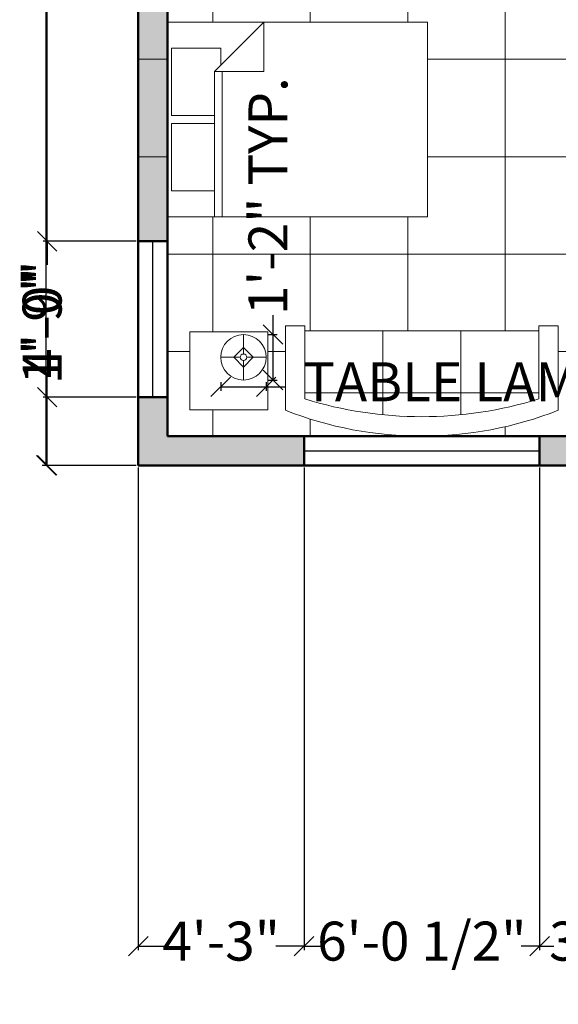
# Model space of a CAD drawing. Units: inches. Extents: x 2371 to 3019, y 129 to 700.
# Tile 1 of 14: x 2371 to 2536, y 129 to 432. Entities that reach past the tile are written whole.
import ezdxf

# ---------------------------------------------------------------- set-up
doc = ezdxf.new("R2010")
doc.units = ezdxf.units.IN
for name, color, linetype, lineweight in [('A-ANNO-DIMS', 2, 'Continuous', 18), ('A-FLOR-PATT', 252, 'Continuous', 13), ('A-FURN', 8, 'Continuous', 18), ('A-GLAZ', 4, 'Continuous', 25), ('A-WALL', 7, 'Continuous', 50), ('A-WALL-PATT', 8, 'Continuous', 13)]:
    doc.layers.add(name, color=color, linetype=linetype, lineweight=lineweight)
doc.styles.get("Standard").update_dxf_attribs({"font": 'arial.ttf'})
doc.dimstyles.new('ISO-25', dxfattribs={"dimtxt": 12, "dimasz": 6, "dimexe": 1.25, "dimexo": 0.625, "dimtad": 0, "dimdec": 1, "dimlunit": 3, "dimtxsty": 'Standard', "dimblk": 'OBLIQUE', "dimblk1": 'ORIGIN2', "dimblk2": 'OBLIQUE', "dimcen": 2.5, "dimadec": 0, "dimazin": 0, "dimtfac": 1, "dimtdec": 1, "dimtmove": 0, "dimatfit": 3, "dimldrblk": 'OBLIQUE', "dimfxl": 1, "dimarcsym": 0})

# ---------------------------------------------------------------- blocks, each defined once
blk = doc.blocks.new('Sofa - Roundback 7 ft.')
for p, q in [((-12.00002, -32.4421), (-12.00003, -6.5971)), ((11.99997, -32.4421), (11.99998, -6.5971)), ((-36.000027, -34), (-36.000027, -11.4696)), ((35.99998, -34), (35.99998, -11.4696)), ((-35.999844, -13.3819), (35.9998, -13.3819)), ((-36.000027, -32.4421), (35.99998, -32.4421))]:
    blk.add_line(p, q)
for points in [[(-36.000027, -34), (-42.000027, -34), (-42.000027, -8)], [(41.99998, -8), (41.99998, -34), (35.99998, -34)]]:
    blk.add_lwpolyline(points)
for centre, radius, start, end in [((0, -114.25), 114.25, 68.43141, 111.5686), ((-0.00001, -127.1968), 121.1968, 72.72033, 107.2797)]:
    blk.add_arc(centre, radius, start, end)
blk = doc.blocks.new('Lamp - Table')
for p, q in [((0, 7), (0, 1)), ((-1, 0), (-7, 0)), ((0, 3), (-3, 0)), ((-3, 0), (0, -3)), ((3, 0), (0, 3)), ((0, -3), (3, 0)), ((1, 0), (7, 0)), ((0, -1), (0, -7))]:
    blk.add_line(p, q)
for radius in [7, 1]:
    blk.add_circle((0, 0), radius)
blk = doc.blocks.new('Bed - Queen')
for p, q in [((0, -80.00003), (0, 0)), ((0, 0), (59.99999, 0)), ((59.99999, 0), (59.99999, -80.00003)), ((7.99999, -1.2), (28.79998, -1.2)), ((7.99999, -14.4), (7.99999, -1.2)), ((28.79998, -1.2), (28.79998, -14.4)), ((31.19999, -1.2), (51.99999, -1.2)), ((31.19999, -14.4), (31.19999, -1.2)), ((51.99999, -1.2), (51.99999, -16.4)), ((0, -14.4), (44.8, -14.4)), ((59.99999, -29.6), (44.8, -14.4)), ((44.8, -14.4), (44.8, -29.6)), ((44.8, -16.8), (0, -16.8)), ((51.99999, -16.4), (46.79936, -16.4)), ((44.8, -29.6), (59.99999, -29.6)), ((59.99999, -80.00003), (0, -80.00003))]:
    blk.add_line(p, q)
blk = doc.blocks.new('_Oblique')
at = {"color": 0, "linetype": 'ByBlock', "lineweight": -2}
blk.add_line((-0.5, -0.5), (0.5, 0.5), dxfattribs=at)
blk = doc.blocks.new('*D18')
at = {"layer": 'A-ANNO-DIMS', "color": 0, "lineweight": -2, "transparency": 16777216}
for p, q in [((2406.48, 630.98), (2377.53, 630.98)), ((2378.78, 630.98), (2378.78, 484.31)), ((2378.78, 294.98), (2378.78, 441.64)), ((2406.48, 294.98), (2377.53, 294.98))]:
    blk.add_line(p, q, dxfattribs=at)
at = {"layer": 'Defpoints', "color": 0, "lineweight": 25, "transparency": 16777216}
for p in [(2407.11, 630.98), (2378.78, 294.98), (2407.11, 294.98)]:
    blk.add_point(p, dxfattribs=at)
at = {"layer": 'A-ANNO-DIMS', "color": 0, "lineweight": -2, "transparency": 16777216, "xscale": 6, "yscale": 6, "zscale": 6}
for p, rotation in [((2378.78, 630.98), 90), ((2378.78, 294.98), 270)]:
    blk.add_blockref('_Oblique', p, dxfattribs=dict(at, rotation=rotation))
at = {"layer": 'A-ANNO-DIMS', "color": 0, "transparency": 16777216, "insert": (2378.78, 462.98), "char_height": 12, "attachment_point": 5, "rotation": 90}
blk.add_mtext('28\'-0"', dxfattribs=at)
blk = doc.blocks.new('_Origin2')
at = {"color": 0, "linetype": 'ByBlock', "lineweight": -2}
blk.add_line((-0.5, 0), (-1, 0), dxfattribs=at)
for radius in [0.5, 0.25]:
    blk.add_circle((0, 0), radius, dxfattribs=at)
blk = doc.blocks.new('*D22')
at = {"layer": 'A-ANNO-DIMS', "color": 0, "lineweight": -2, "transparency": 16777216}
for p, q in [((2432.46, 320.64), (2432.46, 317.92)), ((2432.46, 319.17), (2446.46, 319.17)), ((2446.46, 320.64), (2446.46, 317.92)), ((2446.46, 319.17), (2452.46, 319.17))]:
    blk.add_line(p, q, dxfattribs=at)
at = {"layer": 'Defpoints', "color": 0, "lineweight": 25, "transparency": 16777216}
for p in [(2432.46, 321.27), (2446.46, 321.27), (2446.46, 319.17)]:
    blk.add_point(p, dxfattribs=at)
at = {"layer": 'A-ANNO-DIMS', "color": 0, "lineweight": -2, "transparency": 16777216, "xscale": 6, "yscale": 6, "zscale": 6, "rotation": 180}
blk.add_blockref('_Oblique', (2432.46, 319.17), dxfattribs=at)
at = {"layer": 'A-ANNO-DIMS', "color": 0, "lineweight": -2, "transparency": 16777216, "xscale": 6, "yscale": 6, "zscale": 6}
blk.add_blockref('_Oblique', (2446.46, 319.17), dxfattribs=at)
at = {"layer": 'A-ANNO-DIMS', "color": 0, "transparency": 16777216, "insert": (2543.85, 319.17), "char_height": 12, "attachment_point": 5}
blk.add_mtext('TABLE LAMP 1\'-2" TYP.', dxfattribs=at)
blk = doc.blocks.new('*D23')
at = {"layer": 'A-ANNO-DIMS', "color": 0, "lineweight": -2, "transparency": 16777216}
for p, q in [((2448.56, 335.27), (2448.56, 341.27)), ((2447.08, 335.27), (2449.81, 335.27)), ((2448.56, 321.27), (2448.56, 335.27)), ((2447.08, 321.27), (2449.81, 321.27))]:
    blk.add_line(p, q, dxfattribs=at)
at = {"layer": 'Defpoints', "color": 0, "lineweight": 25, "transparency": 16777216}
for p in [(2446.46, 335.27), (2448.56, 335.27), (2446.46, 321.27)]:
    blk.add_point(p, dxfattribs=at)
at = {"layer": 'A-ANNO-DIMS', "color": 0, "lineweight": -2, "transparency": 16777216, "xscale": 6, "yscale": 6, "zscale": 6}
for p, rotation in [((2448.56, 335.27), 90), ((2448.56, 321.27), 270)]:
    blk.add_blockref('_Oblique', p, dxfattribs=dict(at, rotation=rotation))
at = {"layer": 'A-ANNO-DIMS', "color": 0, "transparency": 16777216, "insert": (2448.56, 377.9), "char_height": 12, "attachment_point": 5, "rotation": 90}
blk.add_mtext('1\'-2" TYP.', dxfattribs=at)
blk = doc.blocks.new('*D50')
at = {"layer": 'A-ANNO-DIMS', "color": 0, "lineweight": -2, "transparency": 16777216}
for p, q in [((2407.11, 294.35), (2407.11, 145.68)), ((2458.11, 294.35), (2458.11, 145.68)), ((2407.11, 146.93), (2415.79, 146.93)), ((2458.11, 146.93), (2449.42, 146.93))]:
    blk.add_line(p, q, dxfattribs=at)
at = {"layer": 'Defpoints', "color": 0, "lineweight": 25, "transparency": 16777216}
for p in [(2407.11, 294.98), (2458.11, 294.98), (2458.11, 146.93)]:
    blk.add_point(p, dxfattribs=at)
at = {"layer": 'A-ANNO-DIMS', "color": 0, "lineweight": -2, "transparency": 16777216, "xscale": 6, "yscale": 6, "zscale": 6, "rotation": 180}
blk.add_blockref('_Oblique', (2407.11, 146.93), dxfattribs=at)
at = {"layer": 'A-ANNO-DIMS', "color": 0, "lineweight": -2, "transparency": 16777216, "xscale": 6, "yscale": 6, "zscale": 6}
blk.add_blockref('_Oblique', (2458.11, 146.93), dxfattribs=at)
at = {"layer": 'A-ANNO-DIMS', "color": 0, "transparency": 16777216, "insert": (2432.61, 146.93), "char_height": 12, "attachment_point": 5}
blk.add_mtext('4\'-3"', dxfattribs=at)
blk = doc.blocks.new('*D51')
at = {"layer": 'A-ANNO-DIMS', "color": 0, "lineweight": -2, "transparency": 16777216}
for p, q in [((2458.11, 294.35), (2458.11, 145.68)), ((2530.61, 294.35), (2530.61, 145.68)), ((2458.11, 146.93), (2463.77, 146.93)), ((2530.61, 146.93), (2524.94, 146.93))]:
    blk.add_line(p, q, dxfattribs=at)
at = {"layer": 'Defpoints', "color": 0, "lineweight": 25, "transparency": 16777216}
for p in [(2458.11, 294.98), (2530.61, 294.98), (2530.61, 146.93)]:
    blk.add_point(p, dxfattribs=at)
at = {"layer": 'A-ANNO-DIMS', "color": 0, "lineweight": -2, "transparency": 16777216, "xscale": 6, "yscale": 6, "zscale": 6, "rotation": 180}
blk.add_blockref('_Oblique', (2458.11, 146.93), dxfattribs=at)
at = {"layer": 'A-ANNO-DIMS', "color": 0, "lineweight": -2, "transparency": 16777216, "xscale": 6, "yscale": 6, "zscale": 6}
blk.add_blockref('_Oblique', (2530.61, 146.93), dxfattribs=at)
at = {"layer": 'A-ANNO-DIMS', "color": 0, "transparency": 16777216, "insert": (2494.36, 146.93), "char_height": 12, "attachment_point": 5}
blk.add_mtext('6\'-0 1/2"', dxfattribs=at)
blk = doc.blocks.new('*D52')
at = {"layer": 'A-ANNO-DIMS', "color": 0, "lineweight": -2, "transparency": 16777216}
for p, q in [((2530.61, 294.35), (2530.61, 145.68)), ((2572.61, 294.35), (2572.61, 145.68)), ((2530.61, 146.93), (2535.03, 146.93)), ((2572.61, 146.93), (2568.18, 146.93))]:
    blk.add_line(p, q, dxfattribs=at)
at = {"layer": 'Defpoints', "color": 0, "lineweight": 25, "transparency": 16777216}
for p in [(2530.61, 294.98), (2572.61, 294.98), (2572.61, 146.93)]:
    blk.add_point(p, dxfattribs=at)
at = {"layer": 'A-ANNO-DIMS', "color": 0, "lineweight": -2, "transparency": 16777216, "xscale": 6, "yscale": 6, "zscale": 6, "rotation": 180}
blk.add_blockref('_Oblique', (2530.61, 146.93), dxfattribs=at)
at = {"layer": 'A-ANNO-DIMS', "color": 0, "lineweight": -2, "transparency": 16777216, "xscale": 6, "yscale": 6, "zscale": 6}
blk.add_blockref('_Oblique', (2572.61, 146.93), dxfattribs=at)
at = {"layer": 'A-ANNO-DIMS', "color": 0, "transparency": 16777216, "insert": (2551.61, 146.93), "char_height": 12, "attachment_point": 5}
blk.add_mtext('3\'-6"', dxfattribs=at)
blk = doc.blocks.new('*D58')
at = {"layer": 'A-ANNO-DIMS', "color": 0, "lineweight": -2, "transparency": 16777216}
for p, q in [((2379.06, 315.98), (2379.06, 321.98)), ((2406.48, 315.98), (2377.81, 315.98)), ((2379.06, 294.98), (2379.06, 315.98)), ((2406.48, 294.98), (2377.81, 294.98))]:
    blk.add_line(p, q, dxfattribs=at)
at = {"layer": 'Defpoints', "color": 0, "lineweight": 25, "transparency": 16777216}
for p in [(2379.06, 315.98), (2407.11, 315.98), (2407.11, 294.98)]:
    blk.add_point(p, dxfattribs=at)
at = {"layer": 'A-ANNO-DIMS', "color": 0, "lineweight": -2, "transparency": 16777216, "xscale": 6, "yscale": 6, "zscale": 6}
for p, rotation in [((2379.06, 315.98), 90), ((2379.06, 294.98), 270)]:
    blk.add_blockref('_Oblique', p, dxfattribs=dict(at, rotation=rotation))
at = {"layer": 'A-ANNO-DIMS', "color": 0, "transparency": 16777216, "insert": (2379.06, 337.99), "char_height": 12, "attachment_point": 5, "rotation": 90}
blk.add_mtext('1\'-9"', dxfattribs=at)
blk = doc.blocks.new('*D59')
at = {"layer": 'A-ANNO-DIMS', "color": 0, "lineweight": -2, "transparency": 16777216}
for p, q in [((2406.48, 363.98), (2377.81, 363.98)), ((2379.06, 363.98), (2379.06, 356.79)), ((2379.06, 315.98), (2379.06, 323.16)), ((2406.48, 315.98), (2377.81, 315.98))]:
    blk.add_line(p, q, dxfattribs=at)
at = {"layer": 'Defpoints', "color": 0, "lineweight": 25, "transparency": 16777216}
for p in [(2379.06, 363.98), (2407.11, 363.98), (2407.11, 315.98)]:
    blk.add_point(p, dxfattribs=at)
at = {"layer": 'A-ANNO-DIMS', "color": 0, "lineweight": -2, "transparency": 16777216, "xscale": 6, "yscale": 6, "zscale": 6}
for p, rotation in [((2379.06, 363.98), 90), ((2379.06, 315.98), 270)]:
    blk.add_blockref('_Oblique', p, dxfattribs=dict(at, rotation=rotation))
at = {"layer": 'A-ANNO-DIMS', "color": 0, "transparency": 16777216, "insert": (2379.06, 339.98), "char_height": 12, "attachment_point": 5, "rotation": 90}
blk.add_mtext('4\'-0"', dxfattribs=at)
blk = doc.blocks.new('*D60')
at = {"layer": 'A-ANNO-DIMS', "color": 0, "lineweight": -2, "transparency": 16777216}
for p, q in [((2406.48, 630.98), (2377.81, 630.98)), ((2379.06, 630.98), (2379.06, 518.81)), ((2379.06, 363.98), (2379.06, 476.14)), ((2406.48, 363.98), (2377.81, 363.98))]:
    blk.add_line(p, q, dxfattribs=at)
at = {"layer": 'Defpoints', "color": 0, "lineweight": 25, "transparency": 16777216}
for p in [(2379.06, 630.98), (2407.11, 630.98), (2407.11, 363.98)]:
    blk.add_point(p, dxfattribs=at)
at = {"layer": 'A-ANNO-DIMS', "color": 0, "lineweight": -2, "transparency": 16777216, "xscale": 6, "yscale": 6, "zscale": 6}
for p, rotation in [((2379.06, 630.98), 90), ((2379.06, 363.98), 270)]:
    blk.add_blockref('_Oblique', p, dxfattribs=dict(at, rotation=rotation))
at = {"layer": 'A-ANNO-DIMS', "color": 0, "transparency": 16777216, "insert": (2379.06, 497.48), "char_height": 12, "attachment_point": 5, "rotation": 90}
blk.add_mtext('22\'-3"', dxfattribs=at)

msp = doc.modelspace()

# ---------------------------------------------------------------- hatches: boundary and pattern name
at = {"layer": 'A-FLOR-PATT'}
h = msp.add_hatch(dxfattribs=at)
h.set_pattern_fill('_USER', color=256, scale=30, pattern_type=0)
h.set_pattern_definition([(0, (0, 0), (0, 30), [])])
h.paths.add_polyline_path([(2913.11, 498.98), (2827.61, 498.98), (2827.61, 531.98), (2832.11, 531.98), (2832.11, 537.98), (2833.61, 537.98), (2833.61, 605.98), (2818.35, 605.98, -1), (2796.86, 605.98), (2781.61, 605.98), (2781.61, 603.98), (2781.61, 533.98), (2757.61, 533.98), (2757.61, 531.98), (2797.61, 531.98), (2797.61, 522.98), (2757.61, 522.98), (2757.61, 516.98), (2754.59, 516.98), (2772.52, 485.76), (2771.01, 484.89), (2770.98, 484.93, -0.097552), (2757.61, 481.1), (2757.61, 422.48), (2837.61, 422.48), (2837.61, 362.48), (2757.61, 362.48), (2757.61, 303.98), (2835.86, 303.98, -0.09439), (2793.86, 311.98), (2793.86, 337.98), (2799.86, 337.98), (2799.86, 336.42), (2871.86, 336.42), (2871.86, 337.98), (2877.86, 337.98), (2877.86, 311.98, -0.09439), (2835.86, 303.98), (2913.11, 303.98), (2913.11, 383.18), (2904.11, 383.18), (2904.11, 419.18), (2913.11, 419.18)])
h.paths.add_polyline_path([(2788.88, 332.88), (2788.88, 308.88), (2764.88, 308.88), (2764.88, 332.88)], flags=16)
h.paths.add_polyline_path([(2788.4, 325.04, -1), (2774.4, 325.04, -1)], flags=0)
h.paths.add_polyline_path([(2781.4, 328.04), (2784.4, 325.04), (2781.4, 322.04), (2778.4, 325.04)], flags=0)
h.paths.add_polyline_path([(2782.4, 325.04, -1), (2780.4, 325.04, -1)], flags=0)
h.paths.add_polyline_path([(2748.61, 480.99), (2754.51, 480.98, 0.119303), (2770.98, 484.93), (2753.07, 516.1), (2754.59, 516.98), (2748.61, 516.98), (2748.61, 539.98), (2712.61, 539.98), (2665.11, 539.98, -0.09439), (2707.11, 531.98), (2707.11, 505.98), (2701.11, 505.98), (2701.11, 507.53), (2629.11, 507.53), (2629.11, 505.98), (2623.11, 505.98), (2623.11, 531.98, -0.09439), (2665.11, 539.98), (2581.61, 539.98), (2581.61, 522.98), (2581.61, 477.98, -0.131044), (2589.61, 507.98), (2615.61, 507.98), (2615.61, 501.98), (2614.05, 501.98), (2614.05, 453.98), (2615.61, 453.98), (2615.61, 447.98), (2589.61, 447.98, -0.131044), (2581.61, 477.98), (2581.61, 432.98), (2572.61, 432.98, 0.119303), (2556.14, 428.99), (2574.12, 397.85), (2572.61, 396.98), (2578.61, 396.98), (2581.61, 396.98), (2581.61, 390.98), (2748.61, 390.98)])
h.paths.add_polyline_path([(2683.1, 447.25), (2652.43, 447.25), (2652.43, 492.22), (2683.1, 492.22)], flags=16)
h.paths.add_polyline_path([(2682.1, 448.25), (2653.43, 448.25), (2653.43, 491.22), (2682.1, 491.22)], flags=0)
h.paths.add_polyline_path([(2613.58, 512.06), (2589.58, 512.06), (2589.58, 536.06), (2613.58, 536.06)], flags=16)
h.paths.add_polyline_path([(2599.1, 528.22, -1), (2613.1, 528.22, -1)], flags=0)
h.paths.add_polyline_path([(2609.1, 528.22), (2606.1, 525.22), (2603.1, 528.22), (2606.1, 531.22)], flags=0)
h.paths.add_polyline_path([(2607.1, 528.22, -1), (2605.1, 528.22, -1)], flags=0)
h.paths.add_polyline_path([(2581.61, 522.98), (2581.61, 621.98), (2572.61, 621.98), (2572.61, 522.98), (2572.61, 500.98), (2565.85, 500.98), (2565.85, 500.15), (2564.82, 500.15), (2561.16, 500.19), (2561.16, 500.17), (2560.13, 500.3), (2560.22, 500.98), (2556.38, 500.98), (2556.43, 500.22), (2555.4, 500.14), (2555.34, 500.98), (2551.07, 500.98), (2551.07, 500.15), (2550.04, 500.15), (2547.64, 500.19), (2547.64, 500.15), (2546.61, 500.15), (2541.79, 500.22), (2540.72, 500.13), (2540.65, 500.98), (2533.37, 500.98), (2533.37, 500.15), (2532.34, 500.15), (2529.13, 500.21), (2529.12, 500.13), (2528.09, 500.22), (2528.16, 500.98), (2523.23, 500.98), (2523.23, 500.15), (2522.2, 500.15), (2519.8, 500.21), (2519.8, 500.15), (2518.77, 500.15), (2514.45, 500.26), (2514.44, 500.14), (2513.41, 500.22), (2513.47, 500.98), (2509.62, 500.98), (2509.71, 500.3), (2508.69, 500.17), (2508.58, 500.98), (2505.03, 500.98), (2505.03, 500.15), (2503.99, 500.15), (2501.07, 500.29), (2501.07, 500.15), (2500.04, 500.15), (2496.44, 500.37), (2496.44, 500.15), (2495.4, 500.15), (2492.55, 500.41), (2492.18, 500.35), (2492.09, 500.98), (2486.11, 500.98), (2486.11, 524.98), (2486.11, 531.98), (2490.61, 531.98), (2490.61, 537.98), (2492.11, 537.98), (2492.11, 605.98), (2476.85, 605.98, -1), (2455.36, 605.98), (2440.11, 605.98), (2440.11, 533.98), (2416.11, 533.98), (2416.11, 605.98), (2416.11, 621.98), (2536.61, 621.98), (2536.61, 630.98), (2407.11, 630.98), (2407.11, 363.98), (2416.11, 363.98), (2416.11, 431.48), (2496.11, 431.48), (2496.11, 371.48), (2416.11, 371.48), (2416.11, 303.98), (2494.36, 303.98, -0.09439), (2452.36, 311.98), (2452.36, 337.98), (2458.36, 337.98), (2458.36, 336.42), (2530.36, 336.42), (2530.36, 337.98), (2536.36, 337.98), (2536.36, 311.98, -0.09439), (2494.36, 303.98), (2572.61, 303.98), (2572.61, 381.98), (2572.61, 396.98), (2554.61, 428.15), (2556.12, 429.03), (2556.14, 428.99, -0.119303), (2572.61, 432.98), (2578.61, 432.98), (2581.61, 432.98)])
h.paths.add_polyline_path([(2450.11, 500.98), (2444.5, 500.98), (2444.44, 500.14), (2443.41, 500.22), (2443.47, 500.98), (2439.62, 500.98), (2439.71, 500.3), (2438.69, 500.17), (2438.58, 500.98), (2435.02, 500.98), (2435.02, 500.15), (2433.99, 500.15), (2433.99, 500.98), (2431.07, 500.98), (2431.07, 500.15), (2430.04, 500.15), (2430.04, 500.98), (2426.43, 500.98), (2426.43, 500.15), (2425.4, 500.15), (2425.4, 500.98), (2423.13, 500.98), (2423.2, 500.5), (2422.18, 500.35), (2422.09, 500.98), (2416.11, 500.98), (2416.11, 524.98), (2416.11, 531.98), (2450.11, 531.98), (2450.11, 522.98)], flags=16)
h.paths.add_polyline_path([(2449.11, 501.98), (2417.11, 501.98), (2417.11, 522.98), (2417.11, 523.98), (2449.11, 523.98)], flags=0)
h.paths.add_polyline_path([(2420.7, 510.73), (2419.36, 520.07), (2420.38, 520.22), (2421.74, 510.73), (2425.4, 510.73), (2425.4, 520.07), (2426.43, 520.07), (2426.43, 510.73), (2430.04, 510.73), (2430.04, 520.07), (2431.07, 520.07), (2431.07, 510.73), (2433.99, 510.73), (2433.99, 520.07), (2435.02, 520.07), (2435.02, 510.73), (2437.35, 510.73), (2436.18, 519.93), (2437.2, 520.06), (2438.39, 510.73), (2444.17, 510.73), (2444.85, 520.08), (2445.88, 520.01), (2445.21, 510.73)], flags=0)
h.paths.add_polyline_path([(2446.94, 336.11), (2446.94, 312.11), (2422.94, 312.11), (2422.94, 336.11)], flags=16)
h.paths.add_polyline_path([(2446.46, 328.27, -1), (2432.46, 328.27, -1)], flags=0)
h.paths.add_polyline_path([(2439.46, 331.27), (2442.46, 328.27), (2439.46, 325.27), (2436.46, 328.27)], flags=0)
h.paths.add_polyline_path([(2440.46, 328.27, -1), (2438.46, 328.27, -1)], flags=0)
h.paths.add_polyline_path([(2816, 444.88), (2866.87, 444.88), (2866.87, 463.54), (2816, 463.54)], flags=24)
h.paths.add_polyline_path([(2794.21, 558.3), (2833.34, 558.3), (2833.34, 576.96), (2794.21, 576.96)], flags=24)
h.paths.add_polyline_path([(2651.69, 411.53), (2711.04, 411.53), (2711.04, 430.19), (2651.69, 430.19)], flags=24)
h.paths.add_polyline_path([(2494.09, 444.88), (2544.97, 444.88), (2544.97, 463.54), (2494.09, 463.54)], flags=24)
h.paths.add_polyline_path([(2444.55, 565.02), (2483.69, 565.02), (2483.69, 583.68), (2444.55, 583.68)], flags=24)
h = msp.add_hatch(dxfattribs=at)
h.set_pattern_fill('_USER', color=256, scale=30, angle=90, pattern_type=0)
h.set_pattern_definition([(90, (0, 0), (-30, 2e-15), [])])
h.paths.add_polyline_path([(2913.11, 498.98), (2827.61, 498.98), (2827.61, 531.98), (2832.11, 531.98), (2832.11, 537.98), (2833.61, 537.98), (2833.61, 605.98), (2818.35, 605.98, -1), (2796.86, 605.98), (2781.61, 605.98), (2781.61, 603.98), (2781.61, 533.98), (2757.61, 533.98), (2757.61, 531.98), (2797.61, 531.98), (2797.61, 522.98), (2757.61, 522.98), (2757.61, 516.98), (2754.59, 516.98), (2772.52, 485.76), (2771.01, 484.89), (2770.98, 484.93, -0.097552), (2757.61, 481.1), (2757.61, 422.48), (2837.61, 422.48), (2837.61, 362.48), (2757.61, 362.48), (2757.61, 303.98), (2835.86, 303.98, -0.09439), (2793.86, 311.98), (2793.86, 337.98), (2799.86, 337.98), (2799.86, 336.42), (2871.86, 336.42), (2871.86, 337.98), (2877.86, 337.98), (2877.86, 311.98, -0.09439), (2835.86, 303.98), (2913.11, 303.98), (2913.11, 383.18), (2904.11, 383.18), (2904.11, 419.18), (2913.11, 419.18)])
h.paths.add_polyline_path([(2788.88, 332.88), (2788.88, 308.88), (2764.88, 308.88), (2764.88, 332.88)], flags=16)
h.paths.add_polyline_path([(2788.4, 325.04, -1), (2774.4, 325.04, -1)], flags=0)
h.paths.add_polyline_path([(2781.4, 328.04), (2784.4, 325.04), (2781.4, 322.04), (2778.4, 325.04)], flags=0)
h.paths.add_polyline_path([(2782.4, 325.04, -1), (2780.4, 325.04, -1)], flags=0)
h.paths.add_polyline_path([(2748.61, 480.99), (2754.51, 480.98, 0.119303), (2770.98, 484.93), (2753.07, 516.1), (2754.59, 516.98), (2748.61, 516.98), (2748.61, 539.98), (2712.61, 539.98), (2665.11, 539.98, -0.09439), (2707.11, 531.98), (2707.11, 505.98), (2701.11, 505.98), (2701.11, 507.53), (2629.11, 507.53), (2629.11, 505.98), (2623.11, 505.98), (2623.11, 531.98, -0.09439), (2665.11, 539.98), (2581.61, 539.98), (2581.61, 522.98), (2581.61, 477.98, -0.131044), (2589.61, 507.98), (2615.61, 507.98), (2615.61, 501.98), (2614.05, 501.98), (2614.05, 453.98), (2615.61, 453.98), (2615.61, 447.98), (2589.61, 447.98, -0.131044), (2581.61, 477.98), (2581.61, 432.98), (2572.61, 432.98, 0.119303), (2556.14, 428.99), (2574.12, 397.85), (2572.61, 396.98), (2578.61, 396.98), (2581.61, 396.98), (2581.61, 390.98), (2748.61, 390.98)])
h.paths.add_polyline_path([(2683.1, 447.25), (2652.43, 447.25), (2652.43, 492.22), (2683.1, 492.22)], flags=16)
h.paths.add_polyline_path([(2682.1, 448.25), (2653.43, 448.25), (2653.43, 491.22), (2682.1, 491.22)], flags=0)
h.paths.add_polyline_path([(2613.58, 512.06), (2589.58, 512.06), (2589.58, 536.06), (2613.58, 536.06)], flags=16)
h.paths.add_polyline_path([(2599.1, 528.22, -1), (2613.1, 528.22, -1)], flags=0)
h.paths.add_polyline_path([(2609.1, 528.22), (2606.1, 525.22), (2603.1, 528.22), (2606.1, 531.22)], flags=0)
h.paths.add_polyline_path([(2607.1, 528.22, -1), (2605.1, 528.22, -1)], flags=0)
h.paths.add_polyline_path([(2581.61, 522.98), (2581.61, 621.98), (2572.61, 621.98), (2572.61, 522.98), (2572.61, 500.98), (2565.85, 500.98), (2565.85, 500.15), (2564.82, 500.15), (2561.16, 500.19), (2561.16, 500.17), (2560.13, 500.3), (2560.22, 500.98), (2556.38, 500.98), (2556.43, 500.22), (2555.4, 500.14), (2555.34, 500.98), (2551.07, 500.98), (2551.07, 500.15), (2550.04, 500.15), (2547.64, 500.19), (2547.64, 500.15), (2546.61, 500.15), (2541.79, 500.22), (2540.72, 500.13), (2540.65, 500.98), (2533.37, 500.98), (2533.37, 500.15), (2532.34, 500.15), (2529.13, 500.21), (2529.12, 500.13), (2528.09, 500.22), (2528.16, 500.98), (2523.23, 500.98), (2523.23, 500.15), (2522.2, 500.15), (2519.8, 500.21), (2519.8, 500.15), (2518.77, 500.15), (2514.45, 500.26), (2514.44, 500.14), (2513.41, 500.22), (2513.47, 500.98), (2509.62, 500.98), (2509.71, 500.3), (2508.69, 500.17), (2508.58, 500.98), (2505.03, 500.98), (2505.03, 500.15), (2503.99, 500.15), (2501.07, 500.29), (2501.07, 500.15), (2500.04, 500.15), (2496.44, 500.37), (2496.44, 500.15), (2495.4, 500.15), (2492.55, 500.41), (2492.18, 500.35), (2492.09, 500.98), (2486.11, 500.98), (2486.11, 524.98), (2486.11, 531.98), (2490.61, 531.98), (2490.61, 537.98), (2492.11, 537.98), (2492.11, 605.98), (2476.85, 605.98, -1), (2455.36, 605.98), (2440.11, 605.98), (2440.11, 533.98), (2416.11, 533.98), (2416.11, 605.98), (2416.11, 621.98), (2536.61, 621.98), (2536.61, 630.98), (2407.11, 630.98), (2407.11, 363.98), (2416.11, 363.98), (2416.11, 431.48), (2496.11, 431.48), (2496.11, 371.48), (2416.11, 371.48), (2416.11, 303.98), (2494.36, 303.98, -0.09439), (2452.36, 311.98), (2452.36, 337.98), (2458.36, 337.98), (2458.36, 336.42), (2530.36, 336.42), (2530.36, 337.98), (2536.36, 337.98), (2536.36, 311.98, -0.09439), (2494.36, 303.98), (2572.61, 303.98), (2572.61, 381.98), (2572.61, 396.98), (2554.61, 428.15), (2556.12, 429.03), (2556.14, 428.99, -0.119303), (2572.61, 432.98), (2578.61, 432.98), (2581.61, 432.98)])
h.paths.add_polyline_path([(2450.11, 500.98), (2444.5, 500.98), (2444.44, 500.14), (2443.41, 500.22), (2443.47, 500.98), (2439.62, 500.98), (2439.71, 500.3), (2438.69, 500.17), (2438.58, 500.98), (2435.02, 500.98), (2435.02, 500.15), (2433.99, 500.15), (2433.99, 500.98), (2431.07, 500.98), (2431.07, 500.15), (2430.04, 500.15), (2430.04, 500.98), (2426.43, 500.98), (2426.43, 500.15), (2425.4, 500.15), (2425.4, 500.98), (2423.13, 500.98), (2423.2, 500.5), (2422.18, 500.35), (2422.09, 500.98), (2416.11, 500.98), (2416.11, 524.98), (2416.11, 531.98), (2450.11, 531.98), (2450.11, 522.98)], flags=16)
h.paths.add_polyline_path([(2449.11, 501.98), (2417.11, 501.98), (2417.11, 522.98), (2417.11, 523.98), (2449.11, 523.98)], flags=0)
h.paths.add_polyline_path([(2420.7, 510.73), (2419.36, 520.07), (2420.38, 520.22), (2421.74, 510.73), (2425.4, 510.73), (2425.4, 520.07), (2426.43, 520.07), (2426.43, 510.73), (2430.04, 510.73), (2430.04, 520.07), (2431.07, 520.07), (2431.07, 510.73), (2433.99, 510.73), (2433.99, 520.07), (2435.02, 520.07), (2435.02, 510.73), (2437.35, 510.73), (2436.18, 519.93), (2437.2, 520.06), (2438.39, 510.73), (2444.17, 510.73), (2444.85, 520.08), (2445.88, 520.01), (2445.21, 510.73)], flags=0)
h.paths.add_polyline_path([(2446.94, 336.11), (2446.94, 312.11), (2422.94, 312.11), (2422.94, 336.11)], flags=16)
h.paths.add_polyline_path([(2446.46, 328.27, -1), (2432.46, 328.27, -1)], flags=0)
h.paths.add_polyline_path([(2439.46, 331.27), (2442.46, 328.27), (2439.46, 325.27), (2436.46, 328.27)], flags=0)
h.paths.add_polyline_path([(2440.46, 328.27, -1), (2438.46, 328.27, -1)], flags=0)
h.paths.add_polyline_path([(2816, 444.88), (2866.87, 444.88), (2866.87, 463.54), (2816, 463.54)], flags=24)
h.paths.add_polyline_path([(2794.21, 558.3), (2833.34, 558.3), (2833.34, 576.96), (2794.21, 576.96)], flags=24)
h.paths.add_polyline_path([(2651.69, 411.53), (2711.04, 411.53), (2711.04, 430.19), (2651.69, 430.19)], flags=24)
h.paths.add_polyline_path([(2494.09, 444.88), (2544.97, 444.88), (2544.97, 463.54), (2494.09, 463.54)], flags=24)
h.paths.add_polyline_path([(2444.55, 565.02), (2483.69, 565.02), (2483.69, 583.68), (2444.55, 583.68)], flags=24)
at = {"layer": 'A-WALL-PATT'}
h = msp.add_hatch(color=256, dxfattribs=at)
h.dxf.hatch_style = 1
h.paths.add_polyline_path([(2536.61, 630.98), (2407.11, 630.98), (2407.11, 363.98), (2416.11, 363.98), (2416.11, 498.98), (2416.11, 522.98), (2416.11, 531.98), (2416.11, 603.98), (2416.11, 621.98), (2536.61, 621.98)])
h.paths.add_polyline_path([(2630.98, 630.98), (2560.61, 630.98), (2560.61, 621.98), (2630.98, 621.98)])
h.paths.add_polyline_path([(2878.11, 630.98), (2699.23, 630.98), (2699.23, 621.98), (2878.11, 621.98)])
h.paths.add_polyline_path([(2496.61, 621.98), (2492.11, 621.98), (2492.11, 569.98), (2496.61, 569.98)], flags=17)
h.paths.add_polyline_path([(2581.61, 621.98), (2572.61, 621.98), (2572.61, 522.98), (2572.61, 498.98), (2572.61, 432.98), (2578.61, 432.98), (2581.61, 432.98), (2581.61, 522.98)])
h.paths.add_polyline_path([(2572.61, 531.98), (2486.11, 531.98), (2486.11, 522.98), (2572.61, 522.98)])
h.paths.add_polyline_path([(2450.11, 531.98), (2440.11, 531.98), (2416.11, 531.98), (2416.11, 522.98), (2450.11, 522.98)], flags=17)
h.paths.add_polyline_path([(2416.11, 315.98), (2407.11, 315.98), (2407.11, 294.98), (2458.11, 294.98), (2458.11, 303.98), (2416.11, 303.98)])
h.paths.add_polyline_path([(2757.61, 303.98), (2530.61, 303.98), (2530.61, 294.98), (2757.61, 294.98)])
h.paths.add_polyline_path([(2581.61, 381.98), (2605.61, 381.98), (2617.61, 381.98), (2617.61, 390.98), (2581.61, 390.98), (2581.61, 396.98), (2572.61, 396.98), (2572.61, 381.98), (2572.61, 303.98), (2581.61, 303.98)])
h.paths.add_polyline_path([(2757.61, 480.98), (2748.61, 480.98), (2748.61, 381.98), (2748.61, 303.98), (2757.61, 303.98), (2757.61, 381.98), (2757.61, 422.48)])
h.paths.add_polyline_path([(2797.61, 531.98), (2757.61, 531.98), (2757.61, 603.98), (2757.61, 621.98), (2748.61, 621.98), (2748.61, 516.99), (2754.59, 516.98), (2757.61, 516.98), (2757.61, 522.98), (2797.61, 522.98)])
h.paths.add_polyline_path([(2913.11, 531.98), (2827.61, 531.98), (2827.61, 522.98), (2913.11, 522.98)])
h.paths.add_polyline_path([(2923.11, 630.98), (2902.11, 630.98), (2902.11, 621.98), (2914.11, 621.98), (2914.11, 363.98), (2923.11, 363.98)])
h.paths.add_polyline_path([(2923.11, 315.98), (2914.11, 315.98), (2914.11, 303.98), (2866.11, 303.98), (2866.11, 294.98), (2923.11, 294.98)])
h.paths.add_polyline_path([(2793.61, 303.98), (2757.61, 303.98), (2757.61, 294.98), (2793.61, 294.98)])

# ---------------------------------------------------------------- linework, layer by layer
at = {"layer": 'A-FURN'}
msp.add_lwpolyline([(2422.94, 312.11), (2446.94, 312.11), (2446.94, 336.11), (2422.94, 336.11)], close=True, dxfattribs=at)
at = {"layer": 'A-GLAZ'}
for p, q in [((2411.61, 315.98), (2411.61, 363.98)), ((2458.11, 299.48), (2530.61, 299.48))]:
    msp.add_line(p, q, dxfattribs=at)
at = {"layer": 'A-WALL'}
for p, q in [((2407.11, 630.98), (2407.11, 294.98)), ((2416.11, 498.98), (2416.11, 303.98)), ((2407.11, 363.98), (2416.11, 363.98)), ((2407.11, 315.98), (2416.11, 315.98)), ((2416.11, 303.98), (2914.11, 303.98)), ((2458.11, 303.98), (2458.11, 294.98)), ((2530.61, 303.98), (2530.61, 294.98)), ((2407.11, 294.98), (2923.11, 294.98))]:
    msp.add_line(p, q, dxfattribs=at)

# ---------------------------------------------------------------- block references
at = {"layer": 'A-FURN'}
for name, p, rotation in [('Bed - Queen', (2416.11, 371.48), 90), ('Sofa - Roundback 7 ft.', (2494.36, 303.98), 180.0000057391524)]:
    msp.add_blockref(name, p, dxfattribs=dict(at, rotation=rotation))
msp.add_blockref('Lamp - Table', (2439.46, 328.27), dxfattribs=at)

# ---------------------------------------------------------------- dimensions: what is measured, and where the dimension line sits
at = {"layer": 'A-ANNO-DIMS'}
for base, p1, p2, text, override, picture, middle in [((2378.78, 294.98), (2407.11, 630.98), (2407.11, 294.98), '28\'-0"', {"dimclrd": 0, "dimclre": 0, "dimclrt": 0}, '*D18', (2378.78, 462.98)), ((2448.56, 335.27), (2446.46, 321.27), (2446.46, 335.27), '<> TYP.', {"dimdec": 1, "dimrnd": 0, "dimzin": 1, "dimlunit": 4, "dimfrac": 2}, '*D23', (2448.56, 377.9))]:
    dim = msp.add_linear_dim(base=base, p1=p1, p2=p2, angle=90, text=text, dimstyle='ISO-25', override=override, dxfattribs=at)
    dim.commit()
    dim.dimension.update_dxf_attribs({"geometry": picture, "text_midpoint": middle})
for base, p1, p2, picture, middle in [((2379.06, 630.98), (2407.11, 363.98), (2407.11, 630.98), '*D60', (2379.06, 497.48)), ((2379.06, 363.98), (2407.11, 315.98), (2407.11, 363.98), '*D59', (2379.06, 339.98)), ((2379.06, 315.98), (2407.11, 294.98), (2407.11, 315.98), '*D58', (2379.06, 337.99))]:
    dim = msp.add_linear_dim(base=base, p1=p1, p2=p2, angle=90, dimstyle='ISO-25', override={"dimdec": 1, "dimlfac": 1, "dimrnd": 0, "dimzin": 1, "dimdsep": 46, "dimlunit": 4, "dimfrac": 2}, dxfattribs=at)
    dim.commit()
    dim.dimension.update_dxf_attribs({"geometry": picture, "text_midpoint": middle})
dim = msp.add_linear_dim(base=(2446.46, 319.17), p1=(2432.46, 321.27), p2=(2446.46, 321.27), text='TABLE LAMP <> TYP.', dimstyle='ISO-25', override={"dimdec": 1, "dimrnd": 0, "dimzin": 1, "dimlunit": 4, "dimfrac": 2}, dxfattribs=at)
dim.commit()
dim.dimension.update_dxf_attribs({"geometry": '*D22', "text_midpoint": (2543.85, 319.17)})
for base, p1, p2, picture, middle in [((2458.11, 146.93), (2407.11, 294.98), (2458.11, 294.98), '*D50', (2432.61, 146.93)), ((2530.61, 146.93), (2458.11, 294.98), (2530.61, 294.98), '*D51', (2494.36, 146.93)), ((2572.61, 146.93), (2530.61, 294.98), (2572.61, 294.98), '*D52', (2551.61, 146.93))]:
    dim = msp.add_linear_dim(base=base, p1=p1, p2=p2, dimstyle='ISO-25', override={"dimdec": 1, "dimlfac": 1, "dimrnd": 0, "dimzin": 1, "dimdsep": 46, "dimlunit": 4, "dimfrac": 2}, dxfattribs=at)
    dim.commit()
    dim.dimension.update_dxf_attribs({"geometry": picture, "text_midpoint": middle})

doc.saveas('drawing.dxf')
